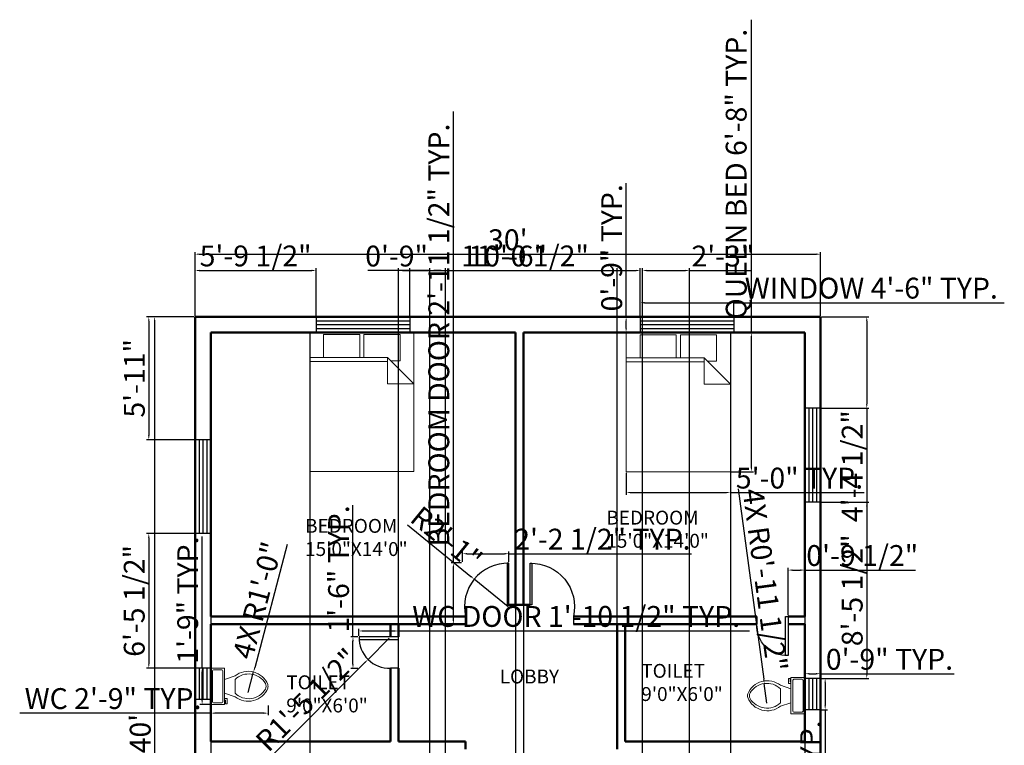
# Model space of a CAD drawing. Units: inches. Extents: x 2787 to 3354, y 1541 to 2259.
# Tile 3 of 3: x 2787 to 3354, y 1842 to 2259. Entities that reach past the tile are written whole.
import ezdxf

# ---------------------------------------------------------------- set-up
doc = ezdxf.new("R2010")
doc.units = ezdxf.units.IN
for name, color, linetype, lineweight in [('A-ANNO-DIMS', 2, 'Continuous', 18), ('A-AREA-IDEN', 7, 'Continuous', 25), ('A-DOOR', 4, 'Continuous', 25), ('A-FLOR-FIXT', 9, 'Continuous', 20), ('A-FURN', 8, 'Continuous', 18), ('A-GLAZ', 4, 'Continuous', 25), ('A-WALL', 7, 'Continuous', 50)]:
    doc.layers.add(name, color=color, linetype=linetype, lineweight=lineweight)
doc.styles.get("Standard").update_dxf_attribs({"font": 'arial.ttf'})
doc.dimstyles.new('ISO-25', dxfattribs={"dimtxt": 12, "dimasz": 2.5, "dimexe": 1.25, "dimexo": 0.625, "dimtad": 1, "dimdec": 1, "dimlunit": 3, "dimtxsty": 'Standard', "dimcen": 2.5, "dimadec": 0, "dimazin": 0, "dimtfac": 1, "dimtdec": 1, "dimtmove": 0, "dimatfit": 3, "dimfxl": 1, "dimarcsym": 0})

# ---------------------------------------------------------------- blocks, each defined once
blk = doc.blocks.new('Bed - Queen')
for p, q in [((0, -80.00003), (0, 0)), ((0, 0), (59.99999, 0)), ((59.99999, 0), (59.99999, -80.00003)), ((7.99999, -1.2), (28.79998, -1.2)), ((7.99999, -14.4), (7.99999, -1.2)), ((28.79998, -1.2), (28.79998, -14.4)), ((31.19999, -1.2), (51.99999, -1.2)), ((31.19999, -14.4), (31.19999, -1.2)), ((51.99999, -1.2), (51.99999, -16.4)), ((0, -14.4), (44.8, -14.4)), ((44.8, -16.8), (0, -16.8)), ((59.99999, -29.6), (44.8, -14.4)), ((44.8, -14.4), (44.8, -29.6)), ((51.99999, -16.4), (46.79936, -16.4)), ((44.8, -29.6), (59.99999, -29.6)), ((59.99999, -80.00003), (0, -80.00003))]:
    blk.add_line(p, q)
blk = doc.blocks.new('Window - Wood Frame 36 in. Wide plan')
for p, q in [((0, 6), (0, 0)), ((0, 4.5), (36, 4.5)), ((36, 6), (36, 0)), ((0, 3), (36, 3)), ((0, 1.5), (36, 1.5))]:
    blk.add_line(p, q)
blk = doc.blocks.new('Toilet - top')
for p, q in [((9.5, -6), (9.5, -2)), ((-10, -8.5), (-8, -8.5)), ((-10, -9.5), (-10, -8.5)), ((-7, -9.5), (-10, -9.5)), ((-8, -8.5), (-8, -8)), ((-7, -8), (-7, -9.5)), ((-4, -8), (-6, -14)), ((4, -8), (6, -14)), ((4, -14), (-4, -14))]:
    blk.add_line(p, q)
blk.add_lwpolyline([(10.5, -8), (10.5, 0), (-10.5, 0), (-10.5, -8)], close=True)
for points in [[(-9.5, -2), (-9.5, -6)], [(8.5, -1), (-8.5, -1)], [(-8.5, -7), (8.5, -7)]]:
    blk.add_lwpolyline(points)
for centre, radius, start, end in [((-8.62, -1.88), 0.884, 81.8699, 188.1301), ((8.62, -1.88), 0.884, 351.8699, 98.1301), ((-8.62, -6.12), 0.884, 171.8699, 278.1301), ((8.62, -6.12), 0.884, 261.8699, 8.1301), ((3.52, -21.58), 12.17, 141.4691, 247.9714), ((4.2, -21.82), 11.33, 136.3677, 238.9468), ((-3.52, -21.58), 12.17, 292.0284, 38.5307), ((-4.2, -21.82), 11.33, 301.053, 43.6321), ((0, -27.88), 4, 245.7318, 294.2682), ((0, -29), 4, 254.8605, 285.1395)]:
    blk.add_arc(centre, radius, start, end)
blk = doc.blocks.new('*D5')
at = {"layer": 'A-ANNO-DIMS', "color": 0, "lineweight": -2, "transparency": 16777216}
for p, q in [((2888.02, 2088.89), (2888.02, 2125.56)), ((3248.02, 2088.89), (3248.02, 2125.56)), ((2890.52, 2124.31), (3245.52, 2124.31))]:
    blk.add_line(p, q, dxfattribs=at)
at = {"layer": 'A-ANNO-DIMS', "color": 0, "transparency": 16777216}
for points in [[(2890.52, 2124.72), (2890.52, 2123.89), (2888.02, 2124.31)], [(3245.52, 2124.72), (3245.52, 2123.89), (3248.02, 2124.31)]]:
    blk.add_solid(points, dxfattribs=at)
at = {"layer": 'Defpoints', "color": 0, "transparency": 16777216}
for p in [(3248.02, 2124.31), (2888.02, 2088.26), (3248.02, 2088.26)]:
    blk.add_point(p, dxfattribs=at)
at = {"layer": 'A-ANNO-DIMS', "color": 0, "transparency": 16777216, "insert": (3068.02, 2131.06), "char_height": 12, "attachment_point": 5}
blk.add_mtext("30'", dxfattribs=at)
blk = doc.blocks.new('*D6')
at = {"layer": 'A-ANNO-DIMS', "color": 0, "lineweight": -2, "transparency": 16777216}
for p, q in [((2887.4, 2088.26), (2863.48, 2088.26)), ((2864.73, 2085.76), (2864.73, 1610.76)), ((2887.4, 1608.26), (2863.48, 1608.26))]:
    blk.add_line(p, q, dxfattribs=at)
at = {"layer": 'A-ANNO-DIMS', "color": 0, "transparency": 16777216}
for points in [[(2864.31, 2085.76), (2865.14, 2085.76), (2864.73, 2088.26)], [(2864.31, 1610.76), (2865.14, 1610.76), (2864.73, 1608.26)]]:
    blk.add_solid(points, dxfattribs=at)
at = {"layer": 'Defpoints', "color": 0, "transparency": 16777216}
for p in [(2888.02, 2088.26), (2864.73, 1608.26), (2888.02, 1608.26)]:
    blk.add_point(p, dxfattribs=at)
at = {"layer": 'A-ANNO-DIMS', "color": 0, "transparency": 16777216, "insert": (2857.97, 1848.26), "char_height": 12, "attachment_point": 5, "rotation": 90}
blk.add_mtext("40'", dxfattribs=at)
blk = doc.blocks.new('DOOR-WC-18IN')
for p, q in [((0, 0), (-18, 0)), ((-18, 0), (-18, -1.5)), ((4.5, 0), (0, 0)), ((-18, -1.5), (4.5, -1.5)), ((4.5, -1.5), (4.5, 0)), ((4.5, -18), (0, -18))]:
    blk.add_line(p, q)
blk.add_arc((-0.75, -0.75), 17.27, 177.5104, 272.4896)
blk = doc.blocks.new('DOOR-BEDROOM-24IN')
for p, q in [((0, 24), (-1, 24)), ((-1, 24), (-1, 0)), ((0, 0), (0, 24)), ((-25, -6.63), (-25, -11.13))]:
    blk.add_line(p, q)
blk.add_arc((-0.5, -1.11), 25.11, 88.8592, 192.6972)
blk = doc.blocks.new('*D12')
at = {"layer": 'A-ANNO-DIMS', "color": 0, "lineweight": -2, "transparency": 16777216}
for p, q in [((3144.24, 2088.89), (3144.24, 2097.61)), ((3198.24, 2088.89), (3198.24, 2097.61)), ((3146.74, 2096.36), (3195.74, 2096.36)), ((3198.24, 2096.36), (3353.84, 2096.36))]:
    blk.add_line(p, q, dxfattribs=at)
at = {"layer": 'A-ANNO-DIMS', "color": 0, "transparency": 16777216}
for points in [[(3146.74, 2096.78), (3146.74, 2095.94), (3144.24, 2096.36)], [(3195.74, 2096.78), (3195.74, 2095.94), (3198.24, 2096.36)]]:
    blk.add_solid(points, dxfattribs=at)
at = {"layer": 'Defpoints', "color": 0, "transparency": 16777216}
for p in [(3198.24, 2096.36), (3144.24, 2088.26), (3198.24, 2088.26)]:
    blk.add_point(p, dxfattribs=at)
at = {"layer": 'A-ANNO-DIMS', "color": 0, "transparency": 16777216, "insert": (3277.29, 2103.19), "char_height": 12, "attachment_point": 5}
blk.add_mtext('WINDOW 4\'-6" TYP.', dxfattribs=at)
blk = doc.blocks.new('*D13')
at = {"layer": 'A-ANNO-DIMS', "color": 0, "lineweight": -2, "transparency": 16777216}
for p, q in [((3136.14, 2088.26), (3136.14, 2165.16)), ((3143.62, 2088.26), (3134.89, 2088.26)), ((3136.14, 2081.76), (3136.14, 2085.76)), ((3143.62, 2079.26), (3134.89, 2079.26))]:
    blk.add_line(p, q, dxfattribs=at)
at = {"layer": 'A-ANNO-DIMS', "color": 0, "transparency": 16777216}
for points in [[(3135.73, 2085.76), (3136.56, 2085.76), (3136.14, 2088.26)], [(3135.73, 2081.76), (3136.56, 2081.76), (3136.14, 2079.26)]]:
    blk.add_solid(points, dxfattribs=at)
at = {"layer": 'Defpoints', "color": 0, "transparency": 16777216}
for p in [(3136.14, 2088.26), (3144.24, 2088.26), (3144.24, 2079.26)]:
    blk.add_point(p, dxfattribs=at)
at = {"layer": 'A-ANNO-DIMS', "color": 0, "transparency": 16777216, "insert": (3129.39, 2127.96), "char_height": 12, "attachment_point": 5, "rotation": 90}
blk.add_mtext('0\'-9" TYP.', dxfattribs=at)
blk = doc.blocks.new('*D14')
at = {"layer": 'A-ANNO-DIMS', "color": 0, "lineweight": -2, "transparency": 16777216}
for p, q in [((3248.65, 1880.03), (3251.97, 1880.03)), ((3250.72, 1877.53), (3250.72, 1864.53)), ((3248.65, 1862.03), (3251.97, 1862.03)), ((3250.72, 1862.03), (3250.72, 1706.43))]:
    blk.add_line(p, q, dxfattribs=at)
at = {"layer": 'A-ANNO-DIMS', "color": 0, "transparency": 16777216}
for points in [[(3250.31, 1877.53), (3251.14, 1877.53), (3250.72, 1880.03)], [(3250.31, 1864.53), (3251.14, 1864.53), (3250.72, 1862.03)]]:
    blk.add_solid(points, dxfattribs=at)
at = {"layer": 'Defpoints', "color": 0, "transparency": 16777216}
for p in [(3248.02, 1880.03), (3248.02, 1862.03), (3250.72, 1862.03)]:
    blk.add_point(p, dxfattribs=at)
at = {"layer": 'A-ANNO-DIMS', "color": 0, "transparency": 16777216, "insert": (3243.89, 1782.98), "char_height": 12, "attachment_point": 5, "rotation": 90}
blk.add_mtext('WINDOW 1\'-6" TYP.', dxfattribs=at)
blk = doc.blocks.new('*D15')
at = {"layer": 'A-ANNO-DIMS', "color": 0, "lineweight": -2, "transparency": 16777216}
for p, q in [((3239.02, 1880.66), (3239.02, 1883.98)), ((3241.52, 1882.73), (3245.52, 1882.73)), ((3248.02, 1880.66), (3248.02, 1883.98)), ((3248.02, 1882.73), (3324.92, 1882.73))]:
    blk.add_line(p, q, dxfattribs=at)
at = {"layer": 'A-ANNO-DIMS', "color": 0, "transparency": 16777216}
for points in [[(3241.52, 1883.15), (3241.52, 1882.32), (3239.02, 1882.73)], [(3245.52, 1883.15), (3245.52, 1882.32), (3248.02, 1882.73)]]:
    blk.add_solid(points, dxfattribs=at)
at = {"layer": 'Defpoints', "color": 0, "transparency": 16777216}
for p in [(3248.02, 1882.73), (3239.02, 1880.03), (3248.02, 1880.03)]:
    blk.add_point(p, dxfattribs=at)
at = {"layer": 'A-ANNO-DIMS', "color": 0, "transparency": 16777216, "insert": (3287.72, 1889.48), "char_height": 12, "attachment_point": 5}
blk.add_mtext('0\'-9" TYP.', dxfattribs=at)
blk = doc.blocks.new('*D16')
at = {"layer": 'A-ANNO-DIMS', "color": 0, "lineweight": -2, "transparency": 16777216}
for p, q in [((3208.24, 2079.05), (3208.24, 2259.33)), ((3196.87, 2079.05), (3209.49, 2079.05)), ((3208.24, 2001.55), (3208.24, 2076.55)), ((3196.87, 1999.05), (3209.49, 1999.05))]:
    blk.add_line(p, q, dxfattribs=at)
at = {"layer": 'A-ANNO-DIMS', "color": 0, "transparency": 16777216}
for points in [[(3207.83, 2076.55), (3208.66, 2076.55), (3208.24, 2079.05)], [(3207.83, 2001.55), (3208.66, 2001.55), (3208.24, 1999.05)]]:
    blk.add_solid(points, dxfattribs=at)
at = {"layer": 'Defpoints', "color": 0, "transparency": 16777216}
for p in [(3196.24, 2079.05), (3208.24, 2079.05), (3196.24, 1999.05)]:
    blk.add_point(p, dxfattribs=at)
at = {"layer": 'A-ANNO-DIMS', "color": 0, "transparency": 16777216, "insert": (3201.05, 2170.44), "char_height": 12, "attachment_point": 5, "rotation": 90}
blk.add_mtext('QUEEN BED 6\'-8" TYP.', dxfattribs=at)
blk = doc.blocks.new('*D17')
at = {"layer": 'A-ANNO-DIMS', "color": 0, "lineweight": -2, "transparency": 16777216}
for p, q in [((3136.24, 1998.43), (3136.24, 1985.8)), ((3196.24, 1998.43), (3196.24, 1985.8)), ((3138.74, 1987.05), (3193.74, 1987.05)), ((3196.24, 1987.05), (3273.14, 1987.05))]:
    blk.add_line(p, q, dxfattribs=at)
at = {"layer": 'A-ANNO-DIMS', "color": 0, "transparency": 16777216}
for points in [[(3138.74, 1987.47), (3138.74, 1986.64), (3136.24, 1987.05)], [(3193.74, 1987.47), (3193.74, 1986.64), (3196.24, 1987.05)]]:
    blk.add_solid(points, dxfattribs=at)
at = {"layer": 'Defpoints', "color": 0, "transparency": 16777216}
for p in [(3136.24, 1999.05), (3196.24, 1999.05), (3196.24, 1987.05)]:
    blk.add_point(p, dxfattribs=at)
at = {"layer": 'A-ANNO-DIMS', "color": 0, "transparency": 16777216, "insert": (3235.94, 1993.81), "char_height": 12, "attachment_point": 5}
blk.add_mtext('5\'-0" TYP.', dxfattribs=at)
blk = doc.blocks.new('*D18')
at = {"layer": 'A-ANNO-DIMS', "color": 0, "lineweight": -2, "transparency": 16777216}
for p, q in [((2897.02, 1860.04), (2787.05, 1860.04)), ((2897.02, 1864.37), (2897.02, 1858.79)), ((2927.57, 1860.04), (2899.52, 1860.04)), ((2930.07, 1864.37), (2930.07, 1858.79))]:
    blk.add_line(p, q, dxfattribs=at)
at = {"layer": 'A-ANNO-DIMS', "color": 0, "transparency": 16777216}
for points in [[(2899.52, 1860.45), (2899.52, 1859.62), (2897.02, 1860.04)], [(2927.57, 1860.45), (2927.57, 1859.62), (2930.07, 1860.04)]]:
    blk.add_solid(points, dxfattribs=at)
at = {"layer": 'Defpoints', "color": 0, "transparency": 16777216}
for p in [(2897.02, 1864.99), (2930.07, 1864.99), (2897.02, 1860.04)]:
    blk.add_point(p, dxfattribs=at)
at = {"layer": 'A-ANNO-DIMS', "color": 0, "transparency": 16777216, "insert": (2840.79, 1866.87), "char_height": 12, "attachment_point": 5}
blk.add_mtext('WC 2\'-9" TYP.', dxfattribs=at)
blk = doc.blocks.new('*D19')
at = {"layer": 'A-ANNO-DIMS', "color": 0, "lineweight": -2, "transparency": 16777216}
for p, q in [((2892.07, 1885.99), (2892.07, 1961.76)), ((2896.4, 1885.99), (2890.82, 1885.99)), ((2892.07, 1867.49), (2892.07, 1883.49)), ((2896.4, 1864.99), (2890.82, 1864.99))]:
    blk.add_line(p, q, dxfattribs=at)
at = {"layer": 'A-ANNO-DIMS', "color": 0, "transparency": 16777216}
for points in [[(2891.65, 1883.49), (2892.48, 1883.49), (2892.07, 1885.99)], [(2891.65, 1867.49), (2892.48, 1867.49), (2892.07, 1864.99)]]:
    blk.add_solid(points, dxfattribs=at)
at = {"layer": 'Defpoints', "color": 0, "transparency": 16777216}
for p in [(2892.07, 1885.99), (2897.02, 1885.99), (2897.02, 1864.99)]:
    blk.add_point(p, dxfattribs=at)
at = {"layer": 'A-ANNO-DIMS', "color": 0, "transparency": 16777216, "insert": (2885.32, 1925.13), "char_height": 12, "attachment_point": 5, "rotation": 90}
blk.add_mtext('1\'-9" TYP.', dxfattribs=at)
blk = doc.blocks.new('*D20')
at = {"layer": 'A-ANNO-DIMS', "color": 0, "lineweight": -2, "transparency": 16777216}
for p, q in [((2982.31, 1904.56), (2982.31, 1908.59)), ((2984.81, 1907.34), (3002.52, 1907.34)), ((3005.02, 1904.56), (3005.02, 1908.59)), ((3005.02, 1907.34), (3207.23, 1907.34))]:
    blk.add_line(p, q, dxfattribs=at)
at = {"layer": 'A-ANNO-DIMS', "color": 0, "transparency": 16777216}
for points in [[(2984.81, 1907.76), (2984.81, 1906.92), (2982.31, 1907.34)], [(3002.52, 1907.76), (3002.52, 1906.92), (3005.02, 1907.34)]]:
    blk.add_solid(points, dxfattribs=at)
at = {"layer": 'Defpoints', "color": 0, "transparency": 16777216}
for p in [(3005.02, 1907.34), (2982.31, 1903.93), (3005.02, 1903.93)]:
    blk.add_point(p, dxfattribs=at)
at = {"layer": 'A-ANNO-DIMS', "color": 0, "transparency": 16777216, "insert": (3107.38, 1914.17), "char_height": 12, "attachment_point": 5}
blk.add_mtext('WC DOOR 1\'-10 1/2" TYP.', dxfattribs=at)
blk = doc.blocks.new('*D21')
at = {"layer": 'A-ANNO-DIMS', "color": 0, "lineweight": -2, "transparency": 16777216}
for p, q in [((2978.91, 1903.93), (2978.91, 1979.7)), ((2981.69, 1903.93), (2977.66, 1903.93)), ((2978.91, 1888.22), (2978.91, 1901.43)), ((2981.69, 1885.72), (2977.66, 1885.72))]:
    blk.add_line(p, q, dxfattribs=at)
at = {"layer": 'A-ANNO-DIMS', "color": 0, "transparency": 16777216}
for points in [[(2978.49, 1901.43), (2979.32, 1901.43), (2978.91, 1903.93)], [(2978.49, 1888.22), (2979.32, 1888.22), (2978.91, 1885.72)]]:
    blk.add_solid(points, dxfattribs=at)
at = {"layer": 'Defpoints', "color": 0, "transparency": 16777216}
for p in [(2978.91, 1903.93), (2982.31, 1903.93), (2982.31, 1885.72)]:
    blk.add_point(p, dxfattribs=at)
at = {"layer": 'A-ANNO-DIMS', "color": 0, "transparency": 16777216, "insert": (2972.16, 1943.07), "char_height": 12, "attachment_point": 5, "rotation": 90}
blk.add_mtext('1\'-6" TYP.', dxfattribs=at)
blk = doc.blocks.new('*D22')
at = {"layer": 'A-ANNO-DIMS', "color": 0, "lineweight": -2, "transparency": 16777216}
for p, q in [((3036.7, 1946.54), (3036.7, 2206.42)), ((3041.37, 1946.54), (3035.45, 1946.54)), ((3036.7, 1913.76), (3036.7, 1944.04)), ((3041.37, 1911.26), (3035.45, 1911.26))]:
    blk.add_line(p, q, dxfattribs=at)
at = {"layer": 'A-ANNO-DIMS', "color": 0, "transparency": 16777216}
for points in [[(3036.29, 1944.04), (3037.12, 1944.04), (3036.7, 1946.54)], [(3036.29, 1913.76), (3037.12, 1913.76), (3036.7, 1911.26)]]:
    blk.add_solid(points, dxfattribs=at)
at = {"layer": 'Defpoints', "color": 0, "transparency": 16777216}
for p in [(3036.7, 1946.54), (3042, 1946.54), (3042, 1911.26)]:
    blk.add_point(p, dxfattribs=at)
at = {"layer": 'A-ANNO-DIMS', "color": 0, "transparency": 16777216, "insert": (3029.87, 2077.73), "char_height": 12, "attachment_point": 5, "rotation": 90}
blk.add_mtext('BEDROOM DOOR 2\'-11 1/2" TYP.', dxfattribs=at)
blk = doc.blocks.new('*D23')
at = {"layer": 'A-ANNO-DIMS', "color": 0, "lineweight": -2, "transparency": 16777216}
for p, q in [((3042, 1947.17), (3042, 1953.09)), ((3044.5, 1951.84), (3066.19, 1951.84)), ((3068.69, 1947.17), (3068.69, 1953.09)), ((3068.69, 1951.84), (3173.76, 1951.84))]:
    blk.add_line(p, q, dxfattribs=at)
at = {"layer": 'A-ANNO-DIMS', "color": 0, "transparency": 16777216}
for points in [[(3044.5, 1952.25), (3044.5, 1951.42), (3042, 1951.84)], [(3066.19, 1952.25), (3066.19, 1951.42), (3068.69, 1951.84)]]:
    blk.add_solid(points, dxfattribs=at)
at = {"layer": 'Defpoints', "color": 0, "transparency": 16777216}
for p in [(3068.69, 1951.84), (3042, 1946.54), (3068.69, 1946.54)]:
    blk.add_point(p, dxfattribs=at)
at = {"layer": 'A-ANNO-DIMS', "color": 0, "transparency": 16777216, "insert": (3122.47, 1958.67), "char_height": 12, "attachment_point": 5}
blk.add_mtext('2\'-2 1/2" TYP.', dxfattribs=at)
blk = doc.blocks.new('*D32')
at = {"layer": 'A-ANNO-DIMS', "color": 0, "lineweight": -2, "transparency": 16777216}
for p, q in [((2888.02, 2088.89), (2888.02, 2116.16)), ((2890.52, 2114.91), (2955.2, 2114.91)), ((2957.7, 2088.89), (2957.7, 2116.16))]:
    blk.add_line(p, q, dxfattribs=at)
at = {"layer": 'A-ANNO-DIMS', "color": 0, "transparency": 16777216}
for points in [[(2890.52, 2115.33), (2890.52, 2114.49), (2888.02, 2114.91)], [(2955.2, 2115.33), (2955.2, 2114.49), (2957.7, 2114.91)]]:
    blk.add_solid(points, dxfattribs=at)
at = {"layer": 'Defpoints', "color": 0, "transparency": 16777216}
for p in [(2957.7, 2114.91), (2888.02, 2088.26), (2957.7, 2088.26)]:
    blk.add_point(p, dxfattribs=at)
at = {"layer": 'A-ANNO-DIMS', "color": 0, "transparency": 16777216, "insert": (2922.86, 2121.74), "char_height": 12, "attachment_point": 5}
blk.add_mtext('5\'-9 1/2"', dxfattribs=at)
blk = doc.blocks.new('*D33')
at = {"layer": 'A-ANNO-DIMS', "color": 0, "lineweight": -2, "transparency": 16777216}
for p, q in [((3011.7, 2088.89), (3011.7, 2116.16)), ((3014.2, 2114.91), (3141.74, 2114.91)), ((3144.24, 2088.89), (3144.24, 2116.16))]:
    blk.add_line(p, q, dxfattribs=at)
at = {"layer": 'A-ANNO-DIMS', "color": 0, "transparency": 16777216}
for points in [[(3014.2, 2115.33), (3014.2, 2114.49), (3011.7, 2114.91)], [(3141.74, 2115.33), (3141.74, 2114.49), (3144.24, 2114.91)]]:
    blk.add_solid(points, dxfattribs=at)
at = {"layer": 'Defpoints', "color": 0, "transparency": 16777216}
for p in [(3144.24, 2114.91), (3011.7, 2088.26), (3144.24, 2088.26)]:
    blk.add_point(p, dxfattribs=at)
at = {"layer": 'A-ANNO-DIMS', "color": 0, "transparency": 16777216, "insert": (3077.97, 2121.74), "char_height": 12, "attachment_point": 5}
blk.add_mtext('11\'-0 1/2"', dxfattribs=at)
blk = doc.blocks.new('*D34')
at = {"layer": 'A-ANNO-DIMS', "color": 0, "lineweight": -2, "transparency": 16777216}
for p, q in [((2887.4, 2088.26), (2860.12, 2088.26)), ((2861.37, 2085.76), (2861.37, 2019.94)), ((2887.4, 2017.44), (2860.12, 2017.44))]:
    blk.add_line(p, q, dxfattribs=at)
at = {"layer": 'A-ANNO-DIMS', "color": 0, "transparency": 16777216}
for points in [[(2860.96, 2085.76), (2861.79, 2085.76), (2861.37, 2088.26)], [(2860.96, 2019.94), (2861.79, 2019.94), (2861.37, 2017.44)]]:
    blk.add_solid(points, dxfattribs=at)
at = {"layer": 'Defpoints', "color": 0, "transparency": 16777216}
for p in [(2888.02, 2088.26), (2861.37, 2017.44), (2888.02, 2017.44)]:
    blk.add_point(p, dxfattribs=at)
at = {"layer": 'A-ANNO-DIMS', "color": 0, "transparency": 16777216, "insert": (2854.62, 2052.85), "char_height": 12, "attachment_point": 5, "rotation": 90}
blk.add_mtext('5\'-11"', dxfattribs=at)
blk = doc.blocks.new('*D35')
at = {"layer": 'A-ANNO-DIMS', "color": 0, "lineweight": -2, "transparency": 16777216}
for p, q in [((2887.4, 1963.44), (2860.12, 1963.44)), ((2861.37, 1960.94), (2861.37, 1888.4)), ((2887.4, 1885.9), (2860.12, 1885.9))]:
    blk.add_line(p, q, dxfattribs=at)
at = {"layer": 'A-ANNO-DIMS', "color": 0, "transparency": 16777216}
for points in [[(2860.96, 1960.94), (2861.79, 1960.94), (2861.37, 1963.44)], [(2860.96, 1888.4), (2861.79, 1888.4), (2861.37, 1885.9)]]:
    blk.add_solid(points, dxfattribs=at)
at = {"layer": 'Defpoints', "color": 0, "transparency": 16777216}
for p in [(2888.02, 1963.44), (2861.37, 1885.9), (2888.02, 1885.9)]:
    blk.add_point(p, dxfattribs=at)
at = {"layer": 'A-ANNO-DIMS', "color": 0, "transparency": 16777216, "insert": (2854.54, 1924.67), "char_height": 12, "attachment_point": 5, "rotation": 90}
blk.add_mtext('6\'-5 1/2"', dxfattribs=at)
blk = doc.blocks.new('*D37')
at = {"layer": 'A-ANNO-DIMS', "color": 0, "lineweight": -2, "transparency": 16777216}
for p, q in [((3248.65, 2088.26), (3275.92, 2088.26)), ((3274.67, 2085.76), (3274.67, 2038.05)), ((3248.65, 2035.55), (3275.92, 2035.55)), ((3274.67, 2035.55), (3274.67, 1971.45))]:
    blk.add_line(p, q, dxfattribs=at)
at = {"layer": 'A-ANNO-DIMS', "color": 0, "transparency": 16777216}
for points in [[(3274.26, 2085.76), (3275.09, 2085.76), (3274.67, 2088.26)], [(3274.26, 2038.05), (3275.09, 2038.05), (3274.67, 2035.55)]]:
    blk.add_solid(points, dxfattribs=at)
at = {"layer": 'Defpoints', "color": 0, "transparency": 16777216}
for p in [(3248.02, 2088.26), (3248.02, 2035.55), (3274.67, 2035.55)]:
    blk.add_point(p, dxfattribs=at)
at = {"layer": 'A-ANNO-DIMS', "color": 0, "transparency": 16777216, "insert": (3267.84, 2002.25), "char_height": 12, "attachment_point": 5, "rotation": 90}
blk.add_mtext('4\'-4 1/2"', dxfattribs=at)
blk = doc.blocks.new('*D38')
at = {"layer": 'A-ANNO-DIMS', "color": 0, "lineweight": -2, "transparency": 16777216}
for p, q in [((3248.65, 1981.55), (3275.92, 1981.55)), ((3274.67, 1979.05), (3274.67, 1882.53)), ((3248.65, 1880.03), (3275.92, 1880.03))]:
    blk.add_line(p, q, dxfattribs=at)
at = {"layer": 'A-ANNO-DIMS', "color": 0, "transparency": 16777216}
for points in [[(3274.26, 1979.05), (3275.09, 1979.05), (3274.67, 1981.55)], [(3274.26, 1882.53), (3275.09, 1882.53), (3274.67, 1880.03)]]:
    blk.add_solid(points, dxfattribs=at)
at = {"layer": 'Defpoints', "color": 0, "transparency": 16777216}
for p in [(3248.02, 1981.55), (3248.02, 1880.03), (3274.67, 1880.03)]:
    blk.add_point(p, dxfattribs=at)
at = {"layer": 'A-ANNO-DIMS', "color": 0, "transparency": 16777216, "insert": (3267.84, 1930.79), "char_height": 12, "attachment_point": 5, "rotation": 90}
blk.add_mtext('8\'-5 1/2"', dxfattribs=at)
blk = doc.blocks.new('*D46')
at = {"layer": 'A-ANNO-DIMS', "color": 0, "lineweight": -2, "transparency": 16777216}
for p, q in [((3005.02, 1844.39), (3005.02, 2116.16)), ((3007.52, 2114.91), (3128.52, 2114.91)), ((3131.02, 1839.89), (3131.02, 2116.16))]:
    blk.add_line(p, q, dxfattribs=at)
at = {"layer": 'A-ANNO-DIMS', "color": 0, "transparency": 16777216}
for points in [[(3007.52, 2115.33), (3007.52, 2114.49), (3005.02, 2114.91)], [(3128.52, 2115.33), (3128.52, 2114.49), (3131.02, 2114.91)]]:
    blk.add_solid(points, dxfattribs=at)
at = {"layer": 'Defpoints', "color": 0, "transparency": 16777216}
for p in [(3131.02, 2114.91), (3005.02, 1843.76), (3131.02, 1839.26)]:
    blk.add_point(p, dxfattribs=at)
at = {"layer": 'A-ANNO-DIMS', "color": 0, "transparency": 16777216, "insert": (3068.02, 2121.66), "char_height": 12, "attachment_point": 5}
blk.add_mtext('10\'-6"', dxfattribs=at)
blk = doc.blocks.new('*D47')
at = {"layer": 'A-ANNO-DIMS', "color": 0, "lineweight": -2, "transparency": 16777216}
for p, q in [((3072.52, 2078.64), (3072.52, 1580.36)), ((3077.02, 2078.64), (3077.02, 1580.36)), ((3070.02, 1581.61), (3067.52, 1581.61)), ((3072.52, 1581.61), (3077.02, 1581.61)), ((3079.52, 1581.61), (3143.13, 1581.61))]:
    blk.add_line(p, q, dxfattribs=at)
at = {"layer": 'A-ANNO-DIMS', "color": 0, "transparency": 16777216}
for points in [[(3070.02, 1582.03), (3070.02, 1581.19), (3072.52, 1581.61)], [(3079.52, 1582.03), (3079.52, 1581.19), (3077.02, 1581.61)]]:
    blk.add_solid(points, dxfattribs=at)
at = {"layer": 'Defpoints', "color": 0, "transparency": 16777216}
for p in [(3072.52, 2079.26), (3077.02, 2079.26), (3077.02, 1581.61)]:
    blk.add_point(p, dxfattribs=at)
at = {"layer": 'A-ANNO-DIMS', "color": 0, "transparency": 16777216, "insert": (3112.58, 1588.44), "char_height": 12, "attachment_point": 5}
blk.add_mtext('0\'-4 1/2"', dxfattribs=at)
blk = doc.blocks.new('*D49')
at = {"layer": 'A-ANNO-DIMS', "color": 0, "lineweight": -2, "transparency": 16777216}
for p, q in [((3023.1, 2114.91), (2987.45, 2114.91)), ((3023.1, 1800.89), (3023.1, 2116.16)), ((3029.6, 2114.91), (3025.6, 2114.91)), ((3032.1, 1796.89), (3032.1, 2116.16))]:
    blk.add_line(p, q, dxfattribs=at)
at = {"layer": 'A-ANNO-DIMS', "color": 0, "transparency": 16777216}
for points in [[(3025.6, 2115.33), (3025.6, 2114.49), (3023.1, 2114.91)], [(3029.6, 2115.33), (3029.6, 2114.49), (3032.1, 2114.91)]]:
    blk.add_solid(points, dxfattribs=at)
at = {"layer": 'Defpoints', "color": 0, "transparency": 16777216}
for p in [(3023.1, 2114.91), (3023.1, 1800.26), (3032.1, 1796.26)]:
    blk.add_point(p, dxfattribs=at)
at = {"layer": 'A-ANNO-DIMS', "color": 0, "transparency": 16777216, "insert": (3004.03, 2121.66), "char_height": 12, "attachment_point": 5}
blk.add_mtext('0\'-9"', dxfattribs=at)
blk = doc.blocks.new('*D50')
at = {"layer": 'A-ANNO-DIMS', "color": 0, "lineweight": -2, "transparency": 16777216}
for p, q in [((2897.02, 2078.64), (2897.02, 1580.36)), ((2953.98, 2078.64), (2953.98, 1580.36)), ((2899.52, 1581.61), (2951.48, 1581.61))]:
    blk.add_line(p, q, dxfattribs=at)
at = {"layer": 'A-ANNO-DIMS', "color": 0, "transparency": 16777216}
for points in [[(2899.52, 1582.03), (2899.52, 1581.19), (2897.02, 1581.61)], [(2951.48, 1582.03), (2951.48, 1581.19), (2953.98, 1581.61)]]:
    blk.add_solid(points, dxfattribs=at)
at = {"layer": 'Defpoints', "color": 0, "transparency": 16777216}
for p in [(2897.02, 2079.26), (2953.98, 2079.26), (2953.98, 1581.61)]:
    blk.add_point(p, dxfattribs=at)
at = {"layer": 'A-ANNO-DIMS', "color": 0, "transparency": 16777216, "insert": (2925.5, 1588.36), "char_height": 12, "attachment_point": 5}
blk.add_mtext('4\'-9"', dxfattribs=at)
blk = doc.blocks.new('*D51')
at = {"layer": 'A-ANNO-DIMS', "color": 0, "lineweight": -2, "transparency": 16777216}
for p, q in [((3196.24, 2078.43), (3196.24, 1580.36)), ((3239.02, 2078.64), (3239.02, 1580.36)), ((3198.74, 1581.61), (3236.52, 1581.61))]:
    blk.add_line(p, q, dxfattribs=at)
at = {"layer": 'A-ANNO-DIMS', "color": 0, "transparency": 16777216}
for points in [[(3198.74, 1582.03), (3198.74, 1581.19), (3196.24, 1581.61)], [(3236.52, 1582.03), (3236.52, 1581.19), (3239.02, 1581.61)]]:
    blk.add_solid(points, dxfattribs=at)
at = {"layer": 'Defpoints', "color": 0, "transparency": 16777216}
for p in [(3196.24, 2079.05), (3239.02, 2079.26), (3239.02, 1581.61)]:
    blk.add_point(p, dxfattribs=at)
at = {"layer": 'A-ANNO-DIMS', "color": 0, "transparency": 16777216, "insert": (3217.63, 1588.37), "char_height": 12, "attachment_point": 5}
blk.add_mtext('3\'-7"', dxfattribs=at)
blk = doc.blocks.new('*D52')
at = {"layer": 'A-ANNO-DIMS', "color": 0, "lineweight": -2, "transparency": 16777216}
for p, q in [((3229.39, 1916.39), (3229.39, 1943.66)), ((3231.89, 1942.41), (3236.52, 1942.41)), ((3239.02, 1916.39), (3239.02, 1943.66)), ((3239.02, 1942.41), (3302.63, 1942.41))]:
    blk.add_line(p, q, dxfattribs=at)
at = {"layer": 'A-ANNO-DIMS', "color": 0, "transparency": 16777216}
for points in [[(3231.89, 1942.83), (3231.89, 1941.99), (3229.39, 1942.41)], [(3236.52, 1942.83), (3236.52, 1941.99), (3239.02, 1942.41)]]:
    blk.add_solid(points, dxfattribs=at)
at = {"layer": 'Defpoints', "color": 0, "transparency": 16777216}
for p in [(3239.02, 1942.41), (3229.39, 1915.76), (3239.02, 1915.76)]:
    blk.add_point(p, dxfattribs=at)
at = {"layer": 'A-ANNO-DIMS', "color": 0, "transparency": 16777216, "insert": (3272.08, 1949.24), "char_height": 12, "attachment_point": 5}
blk.add_mtext('0\'-9 1/2"', dxfattribs=at)
blk = doc.blocks.new('*D56')
at = {"layer": 'A-ANNO-DIMS', "color": 0, "lineweight": -2, "transparency": 16777216}
for p, q in [((3145.52, 1731.89), (3145.52, 2116.16)), ((3148.02, 2114.91), (3170.17, 2114.91)), ((3172.67, 1703.14), (3172.67, 2116.16)), ((3172.67, 2114.91), (3208.53, 2114.91))]:
    blk.add_line(p, q, dxfattribs=at)
at = {"layer": 'A-ANNO-DIMS', "color": 0, "transparency": 16777216}
for points in [[(3148.02, 2115.33), (3148.02, 2114.49), (3145.52, 2114.91)], [(3170.17, 2115.33), (3170.17, 2114.49), (3172.67, 2114.91)]]:
    blk.add_solid(points, dxfattribs=at)
at = {"layer": 'Defpoints', "color": 0, "transparency": 16777216}
for p in [(3172.67, 2114.91), (3145.52, 1731.26), (3172.67, 1702.52)]:
    blk.add_point(p, dxfattribs=at)
at = {"layer": 'A-ANNO-DIMS', "color": 0, "transparency": 16777216, "insert": (3191.85, 2121.67), "char_height": 12, "attachment_point": 5}
blk.add_mtext('2\'-3"', dxfattribs=at)
blk = doc.blocks.new('*D60')
at = {"layer": 'A-ANNO-DIMS', "color": 0, "lineweight": -2, "transparency": 16777216}
for p, q in [((3010.29, 1968.55), (3046.8, 1938.74)), ((3068.19, 1921.28), (3048.74, 1937.16))]:
    blk.add_line(p, q, dxfattribs=at)
at = {"layer": 'A-ANNO-DIMS', "color": 0, "transparency": 16777216}
blk.add_solid([(3047.06, 1939.06), (3046.54, 1938.42), (3048.74, 1937.16)], dxfattribs=at)
at = {"layer": 'Defpoints', "color": 0, "transparency": 16777216}
for p in [(3048.74, 1937.16), (3068.19, 1921.28)]:
    blk.add_point(p, dxfattribs=at)
at = {"layer": 'A-ANNO-DIMS', "color": 0, "transparency": 16777216, "insert": (3031.78, 1959.59), "char_height": 12, "attachment_point": 5, "rotation": 320.7785}
blk.add_mtext('R2\'-1"', dxfattribs=at)
blk = doc.blocks.new('*D62')
at = {"layer": 'A-ANNO-DIMS', "color": 0, "lineweight": -2, "transparency": 16777216}
for p, q in [((2999.77, 1903.18), (2987.57, 1890.97)), ((2932.7, 1836.1), (2985.8, 1889.21))]:
    blk.add_line(p, q, dxfattribs=at)
at = {"layer": 'A-ANNO-DIMS', "color": 0, "transparency": 16777216}
blk.add_solid([(2985.5, 1889.5), (2986.09, 1888.91), (2987.57, 1890.97)], dxfattribs=at)
at = {"layer": 'Defpoints', "color": 0, "transparency": 16777216}
for p in [(2999.77, 1903.18), (2987.57, 1890.97)]:
    blk.add_point(p, dxfattribs=at)
at = {"layer": 'A-ANNO-DIMS', "color": 0, "transparency": 16777216, "insert": (2953.53, 1866.6), "char_height": 12, "attachment_point": 5, "rotation": 45.0011}
blk.add_mtext('R1\'-5 1/2"', dxfattribs=at)
blk = doc.blocks.new('*D65')
at = {"layer": 'A-ANNO-DIMS', "color": 0, "lineweight": -2, "transparency": 16777216}
for p, q in [((2940.99, 1957.15), (2922.33, 1886.16)), ((2918.6, 1871.98), (2921.7, 1883.74))]:
    blk.add_line(p, q, dxfattribs=at)
at = {"layer": 'A-ANNO-DIMS', "color": 0, "transparency": 16777216}
blk.add_solid([(2921.93, 1886.27), (2922.74, 1886.06), (2921.7, 1883.74)], dxfattribs=at)
at = {"layer": 'Defpoints', "color": 0, "transparency": 16777216}
for p in [(2921.7, 1883.74), (2918.6, 1871.98)]:
    blk.add_point(p, dxfattribs=at)
at = {"layer": 'A-ANNO-DIMS', "color": 0, "transparency": 16777216, "insert": (2925.45, 1924.58), "char_height": 12, "attachment_point": 5, "rotation": 75.2779}
blk.add_mtext('4X R1\'-0"', dxfattribs=at)
blk = doc.blocks.new('*D66')
at = {"layer": 'A-ANNO-DIMS', "color": 0, "lineweight": -2, "transparency": 16777216}
for p, q in [((3200.61, 1989.25), (3215.36, 1879.56)), ((3217.21, 1865.85), (3215.7, 1877.08))]:
    blk.add_line(p, q, dxfattribs=at)
at = {"layer": 'A-ANNO-DIMS', "color": 0, "transparency": 16777216}
blk.add_solid([(3215.78, 1879.61), (3214.95, 1879.5), (3215.7, 1877.08)], dxfattribs=at)
at = {"layer": 'Defpoints', "color": 0, "transparency": 16777216}
for p in [(3215.7, 1877.08), (3217.21, 1865.85)]:
    blk.add_point(p, dxfattribs=at)
at = {"layer": 'A-ANNO-DIMS', "color": 0, "transparency": 16777216, "insert": (3214.59, 1936.55), "char_height": 12, "attachment_point": 5, "rotation": 277.6575}
blk.add_mtext('4X R0\'-11 1/2"', dxfattribs=at)

msp = doc.modelspace()

# ---------------------------------------------------------------- linework, layer by layer
at = {"layer": 'A-DOOR'}
for p, q in [((3067.69, 1922.39), (3068.69, 1922.39)), ((3081.82, 1922.39), (3069.82, 1922.39))]:
    msp.add_line(p, q, dxfattribs=at)
at = {"layer": 'A-WALL'}
for p, q in [((2888.02, 2088.26), (3248.02, 2088.26)), ((2888.02, 1608.26), (2888.02, 2088.26)), ((3248.02, 2088.26), (3248.02, 1608.26)), ((2897.02, 2079.26), (3072.52, 2079.26)), ((2897.02, 1915.76), (2897.02, 2079.26)), ((3072.52, 1922.39), (3072.52, 2079.26)), ((3077.02, 1922.39), (3077.02, 2079.26)), ((3077.02, 2079.26), (3239.02, 2079.26)), ((3239.02, 2079.26), (3239.02, 1915.76)), ((3067.69, 1922.39), (3077.02, 1922.39)), ((3077.02, 1922.39), (3080.82, 1922.39)), ((2897.02, 1915.76), (3043.69, 1915.76)), ((3105.82, 1915.76), (3211.39, 1915.76)), ((3229.39, 1915.76), (3239.02, 1915.76)), ((2897.02, 1911.26), (3043.69, 1911.26)), ((2897.02, 1843.76), (2897.02, 1911.26)), ((3000.52, 1903.93), (3000.52, 1911.26)), ((3005.02, 1903.93), (3005.02, 1911.26)), ((3105.82, 1911.26), (3211.39, 1911.26)), ((3131.02, 1911.26), (3131.02, 1839.26)), ((3135.52, 1911.26), (3135.52, 1843.76)), ((3229.39, 1911.26), (3239.02, 1911.26)), ((3239.02, 1911.26), (3239.02, 1843.76)), ((3000.52, 1843.76), (3000.52, 1885.93)), ((3005.02, 1843.76), (3005.02, 1885.93)), ((2897.02, 1843.76), (3000.52, 1843.76)), ((3005.02, 1843.76), (3043.69, 1843.76)), ((3043.69, 1843.76), (3043.69, 1839.26)), ((3135.52, 1843.76), (3239.02, 1843.76))]:
    msp.add_line(p, q, dxfattribs=at)

# ---------------------------------------------------------------- block references
at = {"layer": 'A-DOOR'}
for name, p in [('DOOR-BEDROOM-24IN', (3068.69, 1922.39)), ('DOOR-WC-18IN', (3000.52, 1903.93))]:
    msp.add_blockref(name, p, dxfattribs=at)
at = {"layer": 'A-DOOR', "extrusion": (0, 0, -1), "zscale": -1}
msp.add_blockref('DOOR-BEDROOM-24IN', (-3080.82, 1922.39), dxfattribs=at)
at = {"layer": 'A-DOOR', "extrusion": (0, 0, -1), "zscale": -1, "rotation": 89.99999999999918}
msp.add_blockref('DOOR-WC-18IN', (-3229.39, 1911.26), dxfattribs=at)
at = {"layer": 'A-FLOR-FIXT'}
for p, rotation in [((2897.02, 1875.49), 90), ((3239.02, 1870.05), 270)]:
    msp.add_blockref('Toilet - top', p, dxfattribs=dict(at, rotation=rotation))
at = {"layer": 'A-FURN'}
for p in [(2953.98, 2079.26), (3136.24, 2079.05)]:
    msp.add_blockref('Bed - Queen', p, dxfattribs=at)
at = {"layer": 'A-GLAZ', "xscale": 1.5, "yscale": 1.5, "zscale": 1.5}
for p in [(2957.7, 2079.26), (3144.24, 2079.26)]:
    msp.add_blockref('Window - Wood Frame 36 in. Wide plan', p, dxfattribs=at)
at = {"layer": 'A-GLAZ', "yscale": 1.5, "zscale": 1.5, "rotation": 270}
for p, xscale in [((3239.02, 2035.55), 1.5), ((2888.02, 2017.44), 1.5), ((2888.02, 1885.9), 0.5), ((3239.02, 1880.03), 0.5)]:
    msp.add_blockref('Window - Wood Frame 36 in. Wide plan', p, dxfattribs=dict(at, xscale=xscale))

# ---------------------------------------------------------------- texts
at = {"layer": 'A-AREA-IDEN', "char_height": 8, "attachment_point": 1}
for s, width, insert in [('BEDROOM\\P15\'0"X14\'0"', 81.7488, (3124.76, 1976.6)), ('BEDROOM\\P15\'0"X14\'0"', 81.7488, (2951.35, 1971.86)), ('TOILET\\P9\'0"X6\'0"', 81.7488, (3144.87, 1888.37)), ('TOILET\\P9\'0"X6\'0"', 81.7488, (2940.51, 1881.79)), ('LOBBY', 1.6897, (3063.4, 1885.14))]:
    msp.add_mtext_dynamic_manual_height_columns(s, width=width, gutter_width=12.5, heights=[0], dxfattribs=dict(at, insert=insert))

# ---------------------------------------------------------------- dimensions: what is measured, and where the dimension line sits
at = {"layer": 'A-ANNO-DIMS'}
for base, p1, p2, angle, text, picture, middle in [((3208.24, 2079.05), (3196.24, 1999.05), (3196.24, 2079.05), 90, 'QUEEN BED <> TYP.', '*D16', (3201.05, 2170.44)), ((3036.7, 1946.54), (3042, 1911.26), (3042, 1946.54), 90, 'BEDROOM DOOR <> TYP.', '*D22', (3029.87, 2077.73)), ((3136.14, 2088.26), (3144.24, 2079.26), (3144.24, 2088.26), 90, '<> TYP.', '*D13', (3129.39, 2127.96)), ((2978.91, 1903.93), (2982.31, 1885.72), (2982.31, 1903.93), 90, '<> TYP.', '*D21', (2972.16, 1943.07)), ((2892.07, 1885.99), (2897.02, 1864.99), (2897.02, 1885.99), 90, '<> TYP.', '*D19', (2885.32, 1925.13)), ((2897.024, 1860.038), (2930.0702, 1864.9949), (2897.024, 1864.9949), 180, 'WC <> TYP.', '*D18', (2840.7871, 1866.8676)), ((3250.72, 1862.03), (3248.02, 1880.03), (3248.02, 1862.03), 270, 'WINDOW <> TYP.', '*D14', (3243.89, 1782.98))]:
    dim = msp.add_linear_dim(base=base, p1=p1, p2=p2, angle=angle, text=text, dimstyle='ISO-25', override={"dimdec": 1, "dimlfac": 1, "dimrnd": 0, "dimzin": 1, "dimdsep": 46, "dimlunit": 4, "dimfrac": 2}, dxfattribs=at)
    dim.commit()
    dim.dimension.update_dxf_attribs({"geometry": picture, "text_midpoint": middle})
for base, p1, p2, override, picture, middle in [((2957.7, 2114.91), (2888.02, 2088.26), (2957.7, 2088.26), {"dimdec": 1, "dimlfac": 1, "dimrnd": 0, "dimzin": 1, "dimdsep": 46, "dimlunit": 4, "dimfrac": 2}, '*D32', (2922.86, 2121.74)), ((3248.02, 2124.31), (2888.02, 2088.26), (3248.02, 2088.26), {"dimclrd": 0, "dimclre": 0, "dimclrt": 0}, '*D5', (3068.02, 2131.06)), ((3144.24, 2114.91), (3011.7, 2088.26), (3144.24, 2088.26), {"dimdec": 1, "dimlfac": 1, "dimrnd": 0, "dimzin": 1, "dimdsep": 46, "dimlunit": 4, "dimfrac": 2}, '*D33', (3077.97, 2121.74)), ((3023.1, 2114.91), (3032.1, 1796.26), (3023.1, 1800.26), {"dimdec": 1, "dimlfac": 1, "dimrnd": 0, "dimzin": 1, "dimdsep": 46, "dimlunit": 4, "dimfrac": 2}, '*D49', (3004.03, 2121.66)), ((3131.02, 2114.91), (3005.02, 1843.76), (3131.02, 1839.26), {"dimdec": 1, "dimlfac": 1, "dimrnd": 0, "dimzin": 1, "dimdsep": 46, "dimlunit": 4, "dimfrac": 2}, '*D46', (3068.02, 2121.66)), ((3172.6713, 2114.911), (3145.524, 1731.2609), (3172.6713, 1702.5155), {"dimdec": 1, "dimlfac": 1, "dimrnd": 0, "dimzin": 1, "dimdsep": 46, "dimlunit": 4, "dimfrac": 2}, '*D56', (3191.8482, 2121.6669)), ((2953.98, 1581.61), (2897.02, 2079.26), (2953.98, 2079.26), {"dimdec": 1, "dimlfac": 1, "dimrnd": 0, "dimzin": 1, "dimdsep": 46, "dimlunit": 4, "dimfrac": 2}, '*D50', (2925.5, 1588.36)), ((3077.02, 1581.61), (3072.52, 2079.26), (3077.02, 2079.26), {"dimdec": 1, "dimlfac": 1, "dimrnd": 0, "dimzin": 1, "dimdsep": 46, "dimlunit": 4, "dimfrac": 2}, '*D47', (3112.58, 1588.44)), ((3239.02, 1581.61), (3196.24, 2079.05), (3239.02, 2079.26), {"dimdec": 1, "dimlfac": 1, "dimrnd": 0, "dimzin": 1, "dimdsep": 46, "dimlunit": 4, "dimfrac": 2}, '*D51', (3217.63, 1588.37)), ((3239.02, 1942.41), (3229.39, 1915.76), (3239.02, 1915.76), {"dimdec": 1, "dimlfac": 1, "dimrnd": 0, "dimzin": 1, "dimdsep": 46, "dimlunit": 4, "dimfrac": 2}, '*D52', (3272.08, 1949.24))]:
    dim = msp.add_linear_dim(base=base, p1=p1, p2=p2, dimstyle='ISO-25', override=override, dxfattribs=at)
    dim.commit()
    dim.dimension.update_dxf_attribs({"geometry": picture, "text_midpoint": middle})
for base, p1, p2, text, picture, middle in [((3198.24, 2096.36), (3144.24, 2088.26), (3198.24, 2088.26), 'WINDOW <> TYP.', '*D12', (3277.29, 2103.19)), ((3196.24, 1987.05), (3136.24, 1999.05), (3196.24, 1999.05), '<> TYP.', '*D17', (3235.94, 1993.81)), ((3068.69, 1951.84), (3042, 1946.54), (3068.69, 1946.54), '<> TYP.', '*D23', (3122.47, 1958.67)), ((3005.02, 1907.34), (2982.31, 1903.93), (3005.02, 1903.93), 'WC DOOR <> TYP.', '*D20', (3107.38, 1914.17)), ((3248.02, 1882.73), (3239.02, 1880.03), (3248.02, 1880.03), '<> TYP.', '*D15', (3287.72, 1889.48))]:
    dim = msp.add_linear_dim(base=base, p1=p1, p2=p2, text=text, dimstyle='ISO-25', override={"dimdec": 1, "dimlfac": 1, "dimrnd": 0, "dimzin": 1, "dimdsep": 46, "dimlunit": 4, "dimfrac": 2}, dxfattribs=at)
    dim.commit()
    dim.dimension.update_dxf_attribs({"geometry": picture, "text_midpoint": middle})
for base, p1, p2, override, picture, middle in [((2861.37, 2017.44), (2888.02, 2088.26), (2888.02, 2017.44), {"dimdec": 1, "dimlfac": 1, "dimrnd": 0, "dimzin": 1, "dimdsep": 46, "dimlunit": 4, "dimfrac": 2}, '*D34', (2854.62, 2052.85)), ((2864.73, 1608.26), (2888.02, 2088.26), (2888.02, 1608.26), {"dimclrd": 0, "dimclre": 0, "dimclrt": 0}, '*D6', (2857.97, 1848.26)), ((3274.67, 2035.55), (3248.02, 2088.26), (3248.02, 2035.55), {"dimdec": 1, "dimlfac": 1, "dimrnd": 0, "dimzin": 1, "dimdsep": 46, "dimlunit": 4, "dimfrac": 2}, '*D37', (3267.84, 2002.25)), ((3274.67, 1880.03), (3248.02, 1981.55), (3248.02, 1880.03), {"dimdec": 1, "dimlfac": 1, "dimrnd": 0, "dimzin": 1, "dimdsep": 46, "dimlunit": 4, "dimfrac": 2}, '*D38', (3267.84, 1930.79)), ((2861.37, 1885.9), (2888.02, 1963.44), (2888.02, 1885.9), {"dimdec": 1, "dimlfac": 1, "dimrnd": 0, "dimzin": 1, "dimdsep": 46, "dimlunit": 4, "dimfrac": 2}, '*D35', (2854.54, 1924.67))]:
    dim = msp.add_linear_dim(base=base, p1=p1, p2=p2, angle=90, dimstyle='ISO-25', override=override, dxfattribs=at)
    dim.commit()
    dim.dimension.update_dxf_attribs({"geometry": picture, "text_midpoint": middle})
for center, mpoint, picture, middle in [((3217.21, 1865.85), (3215.7, 1877.08), '*D66', (3214.59, 1936.55)), ((2918.6, 1871.98), (2921.7, 1883.74), '*D65', (2925.45, 1924.58))]:
    dim = msp.add_radius_dim(center=center, mpoint=mpoint, text='4X <>', dimstyle='ISO-25', override={"dimdec": 1, "dimlfac": 1, "dimrnd": 0, "dimzin": 1, "dimdsep": 46, "dimlunit": 4, "dimfrac": 2}, dxfattribs=at)
    dim.commit()
    dim.dimension.update_dxf_attribs({"geometry": picture, "text_midpoint": middle})
for center, mpoint, picture, middle in [((3068.19, 1921.28), (3048.74, 1937.16), '*D60', (3031.78, 1959.59)), ((2999.77, 1903.18), (2987.57, 1890.97), '*D62', (2953.53, 1866.6))]:
    dim = msp.add_radius_dim(center=center, mpoint=mpoint, dimstyle='ISO-25', override={"dimdec": 1, "dimlfac": 1, "dimrnd": 0, "dimzin": 1, "dimdsep": 46, "dimlunit": 4, "dimfrac": 2}, dxfattribs=at)
    dim.commit()
    dim.dimension.update_dxf_attribs({"geometry": picture, "text_midpoint": middle})

doc.saveas('drawing.dxf')
